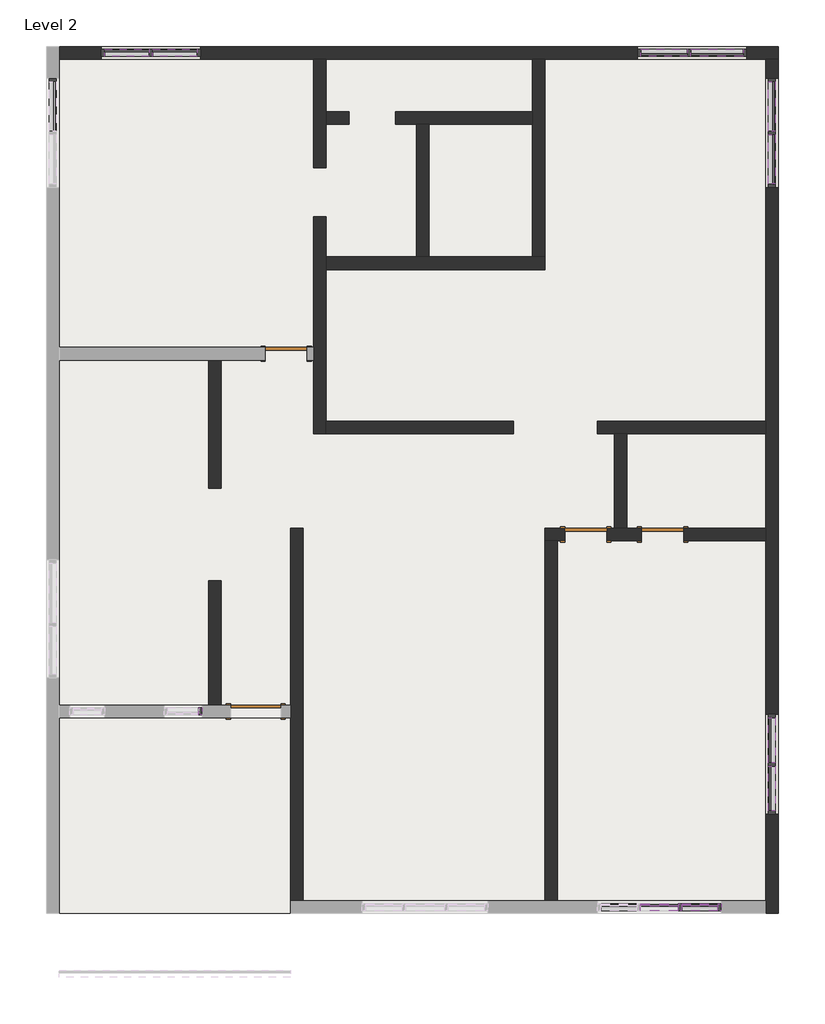
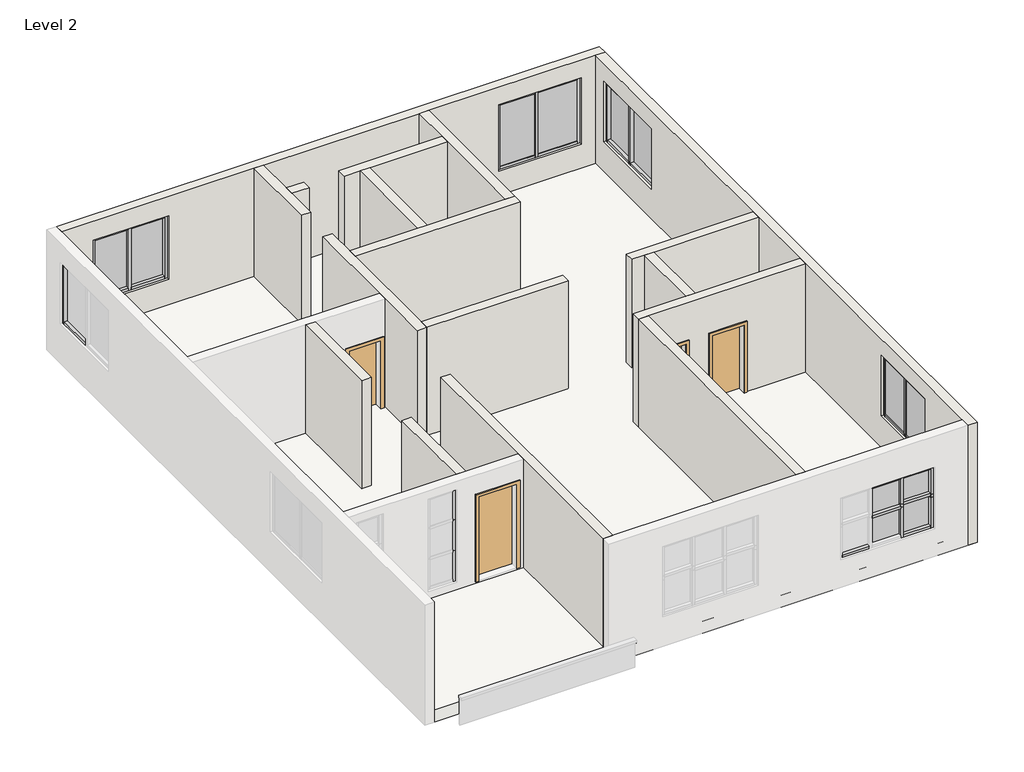
# One storey, part 2 of 2: 45 members, 17 walls, 12 plates, 4 doors, 1 roof.
"""IFC4 building model written with IfcOpenShell, lengths in millimetres."""

from ifc_helpers import new_model, si_unit, frame, origin, place, context, project, spatial, polyline, outline, extrude, faceted_brep, transform, mapped, element, save
from components import door_a1484949, door_85036156, door_0ca8825f, member_00d00b53, member_3d7cb871, member_933cb09f, member_c39a889e, member_9bd02798, member_f1f71bde, member_091e92f8, member_76c917ad, member_e74a93ea, member_cc8ff548, member_70242a31, member_df09edd1, member_4d9a94df, member_b41a733a, member_6d419de8, member_db897065, member_f4ec938c, member_27d1f1c9, member_a044dc63, member_e51dd2bd, member_dfbe4da1, member_32677b83, member_a37bde81, system_panel_glazed_bdc0238d, system_panel_glazed_a6d6e80d, system_panel_glazed_e66cc300, system_panel_glazed_239ce734, system_panel_glazed_acb18a83, system_panel_glazed_af458955, system_panel_glazed_d6f2290d, system_panel_glazed_2cf72723, system_panel_glazed_2eb886e8

model = new_model("IFC4")

# Units and contexts
model_context = context("Model", 3, world=origin())
ifc_project = project(units=[si_unit("LENGTHUNIT", "METRE", prefix="MILLI")], contexts=[model_context])

# Site, building, storey
site = spatial("IfcSite", under=ifc_project)
building = spatial("IfcBuilding", under=site)
storey = spatial("IfcBuildingStorey", under=building, Name="Level 2", Elevation=3048.0)

# Doors
placement = place(None, origin())
door_shape = door_a1484949(model_context)
element("IfcDoor", 1, ObjectType="Single-Flush : 30\" x 80\"", at=placement, inside=storey, context=model_context, shape_type="MappedRepresentation", body=[
    mapped(door_shape, transform((-14457.5127168, -4725.546149, 3048.0), x_axis=(1.0, 0.0, 0.0), y_axis=(0.0, 1.0, 0.0), z_axis=(0.0, 0.0, 1.0))),
])
element("IfcDoor", 2, ObjectType="Single-Flush : 30\" x 80\"", at=placement, inside=storey, context=model_context, shape_type="MappedRepresentation", body=[
    mapped(door_shape, transform((-9027.8261094, -8002.146149, 3048.0), x_axis=(1.0, 0.0, 0.0), y_axis=(0.0, 1.0, 0.0), z_axis=(0.0, 0.0, 1.0))),
])
door_2_shape = door_85036156(model_context)
element("IfcDoor", 3, ObjectType="Single-Flush : 30\" x 80\"", at=placement, inside=storey, context=model_context, shape_type="MappedRepresentation", body=[
    mapped(door_2_shape, transform((-7637.1761094, -8002.146149, 3048.0), x_axis=(-1.0, 0.0, 0.0), y_axis=(0.0, -1.0, 0.0), z_axis=(0.0, 0.0, 1.0))),
])
door_3_shape = door_0ca8825f(model_context)
element("IfcDoor", 4, ObjectType="Single-Flush : 36\" x 84\"", at=placement, inside=storey, context=model_context, shape_type="MappedRepresentation", body=[
    mapped(door_3_shape, transform((-15009.5261094, -11202.546149, 3403.6), x_axis=(1.0, 0.0, 0.0), y_axis=(0.0, 1.0, 0.0), z_axis=(0.0, 0.0, 1.0))),
])

# Members
member_shape = member_00d00b53(model_context)
element("IfcMember", 5, ObjectType="Rectangular Mullion : 2.5\" x 5\" rectangular", at=placement, inside=storey, context=model_context, shape_type="MappedRepresentation", body=[
    mapped(member_shape, transform((-7319.8216452, -14745.846149, 4532.9555732), x_axis=(1.0, 0.0, 0.0), y_axis=(0.0, -1.0, 0.0), z_axis=(0.0, 0.0, -1.0))),
])
member_2_shape = member_3d7cb871(model_context)
element("IfcMember", 6, ObjectType="Rectangular Mullion : 2.5\" x 5\" rectangular", at=placement, inside=storey, context=model_context, shape_type="MappedRepresentation", body=[
    mapped(member_2_shape, transform((-6570.3761094, -14745.846149, 4532.9555732), x_axis=(1.0, 0.0, 0.0), y_axis=(0.0, -1.0, 0.0), z_axis=(0.0, 0.0, -1.0))),
])
member_3_shape = member_933cb09f(model_context)
element("IfcMember", 7, ObjectType="Rectangular Mullion : 2.5\" x 5\" rectangular", at=placement, inside=storey, context=model_context, shape_type="MappedRepresentation", body=[
    mapped(member_3_shape, transform((-5655.9761094, -12194.7225944, 5677.6081175), x_axis=(0.0, 0.0, 1.0), y_axis=(1.0, 0.0, 0.0), z_axis=(0.0, 1.0, 0.0))),
])
element("IfcMember", 8, ObjectType="Rectangular Mullion : 2.5\" x 5\" rectangular", at=placement, inside=storey, context=model_context, shape_type="MappedRepresentation", body=[
    mapped(member_3_shape, transform((-5655.9761094, -11319.9990397, 5677.6081175), x_axis=(0.0, 0.0, 1.0), y_axis=(1.0, 0.0, 0.0), z_axis=(0.0, 1.0, 0.0))),
])
member_4_shape = member_c39a889e(model_context)
element("IfcMember", 9, ObjectType="Rectangular Mullion : 2.5\" x 5\" rectangular", at=placement, inside=storey, context=model_context, shape_type="MappedRepresentation", body=[
    mapped(member_4_shape, transform((-5655.9761094, -12162.9725944, 4144.9262175), x_axis=(0.0, 1.0, 0.0), y_axis=(1.0, 0.0, 0.0), z_axis=(0.0, 0.0, -1.0))),
])
element("IfcMember", 10, ObjectType="Rectangular Mullion : 2.5\" x 5\" rectangular", at=placement, inside=storey, context=model_context, shape_type="MappedRepresentation", body=[
    mapped(member_4_shape, transform((-5655.9761094, -725.046149, 4111.8628556), x_axis=(0.0, -1.0, 0.0), y_axis=(-1.0, 0.0, 0.0), z_axis=(0.0, 0.0, -1.0))),
])
element("IfcMember", 11, ObjectType="Rectangular Mullion : 2.5\" x 5\" rectangular", at=placement, inside=storey, context=model_context, shape_type="MappedRepresentation", body=[
    mapped(member_3_shape, transform((-5655.9761094, -12131.2225944, 4144.9262175), x_axis=(0.0, 0.0, -1.0), y_axis=(1.0, 0.0, 0.0), z_axis=(0.0, -1.0, 0.0))),
])
element("IfcMember", 12, ObjectType="Rectangular Mullion : 2.5\" x 5\" rectangular", at=placement, inside=storey, context=model_context, shape_type="MappedRepresentation", body=[
    mapped(member_3_shape, transform((-5655.9761094, -13005.946149, 4144.9262175), x_axis=(0.0, 0.0, -1.0), y_axis=(1.0, 0.0, 0.0), z_axis=(0.0, -1.0, 0.0))),
])
member_5_shape = member_9bd02798(model_context)
element("IfcMember", 13, ObjectType="Rectangular Mullion : 2.5\" x 5\" rectangular", at=placement, inside=storey, context=model_context, shape_type="MappedRepresentation", body=[
    mapped(member_5_shape, transform((-5655.9761094, -11256.4990397, 4144.9262175), x_axis=(0.0, 1.0, 0.0), y_axis=(1.0, 0.0, 0.0), z_axis=(0.0, 0.0, -1.0))),
])
element("IfcMember", 14, ObjectType="Rectangular Mullion : 2.5\" x 5\" rectangular", at=placement, inside=storey, context=model_context, shape_type="MappedRepresentation", body=[
    mapped(member_5_shape, transform((-5655.9761094, -1715.646149, 4111.8628556), x_axis=(0.0, -1.0, 0.0), y_axis=(-1.0, 0.0, 0.0), z_axis=(0.0, 0.0, -1.0))),
])
element("IfcMember", 15, ObjectType="Rectangular Mullion : 2.5\" x 5\" rectangular", at=placement, inside=storey, context=model_context, shape_type="MappedRepresentation", body=[
    mapped(member_5_shape, transform((-5655.9761094, -13069.446149, 5677.6081175), x_axis=(0.0, -1.0, 0.0), y_axis=(1.0, 0.0, 0.0), z_axis=(0.0, 0.0, 1.0))),
])
element("IfcMember", 16, ObjectType="Rectangular Mullion : 2.5\" x 5\" rectangular", at=placement, inside=storey, context=model_context, shape_type="MappedRepresentation", body=[
    mapped(member_5_shape, transform((-5655.9761094, 265.553851, 5644.5447557), x_axis=(0.0, 1.0, 0.0), y_axis=(-1.0, 0.0, 0.0), z_axis=(0.0, 0.0, 1.0))),
])
member_6_shape = member_f1f71bde(model_context)
element("IfcMember", 17, ObjectType="Rectangular Mullion : 2.5\" x 5\" rectangular", at=placement, inside=storey, context=model_context, shape_type="MappedRepresentation", body=[
    mapped(member_6_shape, transform((-5655.9761094, -756.796149, 4111.8628556), x_axis=(0.0, 0.0, -1.0), y_axis=(-1.0, 0.0, 0.0), z_axis=(0.0, 1.0, 0.0))),
])
element("IfcMember", 18, ObjectType="Rectangular Mullion : 2.5\" x 5\" rectangular", at=placement, inside=storey, context=model_context, shape_type="MappedRepresentation", body=[
    mapped(member_6_shape, transform((-5655.9761094, 202.053851, 4111.8628556), x_axis=(0.0, 0.0, -1.0), y_axis=(-1.0, 0.0, 0.0), z_axis=(0.0, 1.0, 0.0))),
])
element("IfcMember", 19, ObjectType="Rectangular Mullion : 2.5\" x 5\" rectangular", at=placement, inside=storey, context=model_context, shape_type="MappedRepresentation", body=[
    mapped(member_6_shape, transform((-18686.1761094, 202.053851, 4059.4675701), x_axis=(0.0, 0.0, -1.0), y_axis=(-1.0, 0.0, 0.0), z_axis=(0.0, 1.0, 0.0))),
])
element("IfcMember", 20, ObjectType="Rectangular Mullion : 2.5\" x 5\" rectangular", at=placement, inside=storey, context=model_context, shape_type="MappedRepresentation", body=[
    mapped(member_6_shape, transform((-5655.9761094, -693.296149, 5644.5447557), x_axis=(0.0, 0.0, 1.0), y_axis=(-1.0, 0.0, 0.0), z_axis=(0.0, -1.0, 0.0))),
])
element("IfcMember", 21, ObjectType="Rectangular Mullion : 2.5\" x 5\" rectangular", at=placement, inside=storey, context=model_context, shape_type="MappedRepresentation", body=[
    mapped(member_6_shape, transform((-5655.9761094, -1652.146149, 5644.5447557), x_axis=(0.0, 0.0, 1.0), y_axis=(-1.0, 0.0, 0.0), z_axis=(0.0, -1.0, 0.0))),
])
member_7_shape = member_091e92f8(model_context)
element("IfcMember", 22, ObjectType="Rectangular Mullion : 2.5\" x 5\" rectangular", at=placement, inside=storey, context=model_context, shape_type="MappedRepresentation", body=[
    mapped(member_7_shape, transform((-8030.8761094, 722.753851, 5648.4248448), x_axis=(0.0, 0.0, 1.0), y_axis=(0.0, 1.0, 0.0), z_axis=(-1.0, 0.0, 0.0))),
])
member_8_shape = member_76c917ad(model_context)
element("IfcMember", 23, ObjectType="Rectangular Mullion : 2.5\" x 5\" rectangular", at=placement, inside=storey, context=model_context, shape_type="MappedRepresentation", body=[
    mapped(member_8_shape, transform((-7154.5761094, 722.753851, 3961.5338093), x_axis=(-1.0, 0.0, 0.0), y_axis=(0.0, 1.0, 0.0), z_axis=(0.0, 0.0, -1.0))),
])
element("IfcMember", 24, ObjectType="Rectangular Mullion : 2.5\" x 5\" rectangular", at=placement, inside=storey, context=model_context, shape_type="MappedRepresentation", body=[
    mapped(member_7_shape, transform((-7186.3261094, 722.753851, 3961.5338093), x_axis=(0.0, 0.0, -1.0), y_axis=(0.0, 1.0, 0.0), z_axis=(1.0, 0.0, 0.0))),
])
member_9_shape = member_e74a93ea(model_context)
element("IfcMember", 25, ObjectType="Rectangular Mullion : 2.5\" x 5\" rectangular", at=placement, inside=storey, context=model_context, shape_type="MappedRepresentation", body=[
    mapped(member_9_shape, transform((-8094.3761094, 722.753851, 3961.5338093), x_axis=(-1.0, 0.0, 0.0), y_axis=(0.0, 1.0, 0.0), z_axis=(0.0, 0.0, -1.0))),
])
member_10_shape = member_cc8ff548(model_context)
element("IfcMember", 26, ObjectType="Rectangular Mullion : 2.5\" x 5\" rectangular", at=placement, inside=storey, context=model_context, shape_type="MappedRepresentation", body=[
    mapped(member_10_shape, transform((-7122.8261094, 722.753851, 5648.4248448), x_axis=(0.0, 0.0, 1.0), y_axis=(0.0, 1.0, 0.0), z_axis=(-1.0, 0.0, 0.0))),
])
element("IfcMember", 27, ObjectType="Rectangular Mullion : 2.5\" x 5\" rectangular", at=placement, inside=storey, context=model_context, shape_type="MappedRepresentation", body=[
    mapped(member_10_shape, transform((-6176.6761094, 722.753851, 3961.5338093), x_axis=(0.0, 0.0, -1.0), y_axis=(0.0, 1.0, 0.0), z_axis=(1.0, 0.0, 0.0))),
])
element("IfcMember", 28, ObjectType="Rectangular Mullion : 2.5\" x 5\" rectangular", at=placement, inside=storey, context=model_context, shape_type="MappedRepresentation", body=[
    mapped(member_9_shape, transform((-6113.1761094, 722.753851, 5648.4248448), x_axis=(1.0, 0.0, 0.0), y_axis=(0.0, 1.0, 0.0), z_axis=(0.0, 0.0, 1.0))),
])
member_11_shape = member_70242a31(model_context)
element("IfcMember", 29, ObjectType="Rectangular Mullion : 2.5\" x 5\" rectangular", at=placement, inside=storey, context=model_context, shape_type="MappedRepresentation", body=[
    mapped(member_11_shape, transform((-16940.3627168, 722.753851, 5613.602116), x_axis=(0.0, 0.0, 1.0), y_axis=(0.0, -1.0, 0.0), z_axis=(1.0, 0.0, 0.0))),
])
element("IfcMember", 30, ObjectType="Rectangular Mullion : 2.5\" x 5\" rectangular", at=placement, inside=storey, context=model_context, shape_type="MappedRepresentation", body=[
    mapped(member_11_shape, transform((-16070.4127168, 722.753851, 5613.602116), x_axis=(0.0, 0.0, 1.0), y_axis=(0.0, -1.0, 0.0), z_axis=(1.0, 0.0, 0.0))),
])
member_12_shape = member_df09edd1(model_context)
element("IfcMember", 31, ObjectType="Rectangular Mullion : 2.5\" x 5\" rectangular", at=placement, inside=storey, context=model_context, shape_type="MappedRepresentation", body=[
    mapped(member_12_shape, transform((-16908.6127168, 722.753851, 4001.8843583), x_axis=(1.0, 0.0, 0.0), y_axis=(0.0, -1.0, 0.0), z_axis=(0.0, 0.0, -1.0))),
])
element("IfcMember", 32, ObjectType="Rectangular Mullion : 2.5\" x 5\" rectangular", at=placement, inside=storey, context=model_context, shape_type="MappedRepresentation", body=[
    mapped(member_11_shape, transform((-16876.8627168, 722.753851, 4001.8843583), x_axis=(0.0, 0.0, -1.0), y_axis=(0.0, -1.0, 0.0), z_axis=(-1.0, 0.0, 0.0))),
])
element("IfcMember", 33, ObjectType="Rectangular Mullion : 2.5\" x 5\" rectangular", at=placement, inside=storey, context=model_context, shape_type="MappedRepresentation", body=[
    mapped(member_11_shape, transform((-17746.8127168, 722.753851, 4001.8843583), x_axis=(0.0, 0.0, -1.0), y_axis=(0.0, -1.0, 0.0), z_axis=(-1.0, 0.0, 0.0))),
])
member_13_shape = member_4d9a94df(model_context)
element("IfcMember", 34, ObjectType="Rectangular Mullion : 2.5\" x 5\" rectangular", at=placement, inside=storey, context=model_context, shape_type="MappedRepresentation", body=[
    mapped(member_13_shape, transform((-17810.3127168, 722.753851, 5613.602116), x_axis=(-1.0, 0.0, 0.0), y_axis=(0.0, -1.0, 0.0), z_axis=(0.0, 0.0, 1.0))),
])
element("IfcMember", 35, ObjectType="Rectangular Mullion : 2.5\" x 5\" rectangular", at=placement, inside=storey, context=model_context, shape_type="MappedRepresentation", body=[
    mapped(member_13_shape, transform((-16006.9127168, 722.753851, 4001.8843583), x_axis=(1.0, 0.0, 0.0), y_axis=(0.0, -1.0, 0.0), z_axis=(0.0, 0.0, -1.0))),
])
member_14_shape = member_b41a733a(model_context)
element("IfcMember", 36, ObjectType="Rectangular Mullion : 2.5\" x 5\" rectangular", at=placement, inside=storey, context=model_context, shape_type="MappedRepresentation", body=[
    mapped(member_14_shape, transform((-18686.1761094, 265.553851, 5599.1263641), x_axis=(0.0, 1.0, 0.0), y_axis=(-1.0, 0.0, 0.0), z_axis=(0.0, 0.0, 1.0))),
])
member_15_shape = member_6d419de8(model_context)
element("IfcMember", 37, ObjectType="Rectangular Mullion : 2.5\" x 5\" rectangular", at=placement, inside=storey, context=model_context, shape_type="MappedRepresentation", body=[
    mapped(member_15_shape, transform((-15981.0761094, -11202.546149, 5884.8075695), x_axis=(1.0, 0.0, 0.0), y_axis=(0.0, 1.0, 0.0), z_axis=(0.0, 0.0, 1.0))),
])
element("IfcMember", 38, ObjectType="Rectangular Mullion : 2.5\" x 5\" rectangular", at=placement, inside=storey, context=model_context, shape_type="MappedRepresentation", body=[
    mapped(member_15_shape, transform((-15981.0761094, -11202.546149, 5104.8752687), x_axis=(1.0, 0.0, 0.0), y_axis=(0.0, 1.0, 0.0), z_axis=(0.0, 0.0, 1.0))),
])
element("IfcMember", 39, ObjectType="Rectangular Mullion : 2.5\" x 5\" rectangular", at=placement, inside=storey, context=model_context, shape_type="MappedRepresentation", body=[
    mapped(member_15_shape, transform((-15981.0761094, -11202.546149, 4324.942968), x_axis=(1.0, 0.0, 0.0), y_axis=(0.0, 1.0, 0.0), z_axis=(0.0, 0.0, 1.0))),
])
member_16_shape = member_db897065(model_context)
element("IfcMember", 40, ObjectType="Rectangular Mullion : 2.5\" x 5\" rectangular", at=placement, inside=storey, context=model_context, shape_type="MappedRepresentation", body=[
    mapped(member_16_shape, transform((-7319.8216452, -14745.846149, 4609.1555732), x_axis=(1.0, 0.0, 0.0), y_axis=(0.0, -1.0, 0.0), z_axis=(0.0, 0.0, -1.0))),
])
member_17_shape = member_f4ec938c(model_context)
element("IfcMember", 41, ObjectType="Rectangular Mullion : 2.5\" x 5\" rectangular", at=placement, inside=storey, context=model_context, shape_type="MappedRepresentation", body=[
    mapped(member_17_shape, transform((-7351.5716452, -14745.846149, 5311.3816242), x_axis=(0.0, 0.0, 1.0), y_axis=(0.0, -1.0, 0.0), z_axis=(1.0, 0.0, 0.0))),
])
member_18_shape = member_27d1f1c9(model_context)
element("IfcMember", 42, ObjectType="Rectangular Mullion : 2.5\" x 5\" rectangular", at=placement, inside=storey, context=model_context, shape_type="MappedRepresentation", body=[
    mapped(member_18_shape, transform((-7351.5716452, -14745.846149, 4532.9555732), x_axis=(0.0, 0.0, 1.0), y_axis=(0.0, -1.0, 0.0), z_axis=(1.0, 0.0, 0.0))),
])
member_19_shape = member_a044dc63(model_context)
element("IfcMember", 43, ObjectType="Rectangular Mullion : 2.5\" x 5\" rectangular", at=placement, inside=storey, context=model_context, shape_type="MappedRepresentation", body=[
    mapped(member_19_shape, transform((-6633.8761094, -14745.846149, 5311.3816242), x_axis=(0.0, 0.0, 1.0), y_axis=(0.0, -1.0, 0.0), z_axis=(1.0, 0.0, 0.0))),
])
member_20_shape = member_e51dd2bd(model_context)
element("IfcMember", 44, ObjectType="Rectangular Mullion : 2.5\" x 5\" rectangular", at=placement, inside=storey, context=model_context, shape_type="MappedRepresentation", body=[
    mapped(member_20_shape, transform((-6633.8761094, -14745.846149, 4609.1555732), x_axis=(0.0, 0.0, 1.0), y_axis=(0.0, -1.0, 0.0), z_axis=(1.0, 0.0, 0.0))),
])
member_21_shape = member_dfbe4da1(model_context)
element("IfcMember", 45, ObjectType="Rectangular Mullion : 2.5\" x 5\" rectangular", at=placement, inside=storey, context=model_context, shape_type="MappedRepresentation", body=[
    mapped(member_21_shape, transform((-6570.3761094, -14745.846149, 4609.1555732), x_axis=(1.0, 0.0, 0.0), y_axis=(0.0, -1.0, 0.0), z_axis=(0.0, 0.0, -1.0))),
])
member_22_shape = member_32677b83(model_context)
element("IfcMember", 46, ObjectType="Rectangular Mullion : 2.5\" x 5\" rectangular", at=placement, inside=storey, context=model_context, shape_type="MappedRepresentation", body=[
    mapped(member_22_shape, transform((-7319.8216452, -14745.846149, 3754.5295223), x_axis=(1.0, 0.0, 0.0), y_axis=(0.0, -1.0, 0.0), z_axis=(0.0, 0.0, -1.0))),
])
element("IfcMember", 47, ObjectType="Rectangular Mullion : 2.5\" x 5\" rectangular", at=placement, inside=storey, context=model_context, shape_type="MappedRepresentation", body=[
    mapped(member_19_shape, transform((-7288.0716452, -14745.846149, 3754.5295223), x_axis=(0.0, 0.0, -1.0), y_axis=(0.0, -1.0, 0.0), z_axis=(-1.0, 0.0, 0.0))),
])
element("IfcMember", 48, ObjectType="Rectangular Mullion : 2.5\" x 5\" rectangular", at=placement, inside=storey, context=model_context, shape_type="MappedRepresentation", body=[
    mapped(member_19_shape, transform((-8755.2127168, -14745.846149, 3754.5295223), x_axis=(0.0, 0.0, -1.0), y_axis=(0.0, -1.0, 0.0), z_axis=(-1.0, 0.0, 0.0))),
])
member_23_shape = member_a37bde81(model_context)
element("IfcMember", 49, ObjectType="Rectangular Mullion : 2.5\" x 5\" rectangular", at=placement, inside=storey, context=model_context, shape_type="MappedRepresentation", body=[
    mapped(member_23_shape, transform((-6570.3761094, -14745.846149, 3754.5295223), x_axis=(1.0, 0.0, 0.0), y_axis=(0.0, -1.0, 0.0), z_axis=(0.0, 0.0, -1.0))),
])

# Plates
system_panel_glazed_shape = system_panel_glazed_bdc0238d(model_context)
element("IfcPlate", 50, ObjectType="System Panel : Glazed", at=placement, inside=storey, context=model_context, shape_type="MappedRepresentation", body=[
    mapped(system_panel_glazed_shape, transform((-5655.9761094, -12600.3343717, 4208.4262175), x_axis=(0.0, 1.0, 0.0), y_axis=(-1.0, 0.0, 0.0), z_axis=(0.0, 0.0, 1.0))),
])
element("IfcPlate", 51, ObjectType="System Panel : Glazed", at=placement, inside=storey, context=model_context, shape_type="MappedRepresentation", body=[
    mapped(system_panel_glazed_shape, transform((-5655.9761094, -11725.610817, 4208.4262175), x_axis=(0.0, 1.0, 0.0), y_axis=(-1.0, 0.0, 0.0), z_axis=(0.0, 0.0, 1.0))),
])
system_panel_glazed_2_shape = system_panel_glazed_a6d6e80d(model_context)
element("IfcPlate", 52, ObjectType="System Panel : Glazed", at=placement, inside=storey, context=model_context, shape_type="MappedRepresentation", body=[
    mapped(system_panel_glazed_2_shape, transform((-5655.9761094, -245.621149, 4175.3628556), x_axis=(0.0, -1.0, 0.0), y_axis=(1.0, 0.0, 0.0), z_axis=(0.0, 0.0, 1.0))),
])
element("IfcPlate", 53, ObjectType="System Panel : Glazed", at=placement, inside=storey, context=model_context, shape_type="MappedRepresentation", body=[
    mapped(system_panel_glazed_2_shape, transform((-5655.9761094, -1204.471149, 4175.3628556), x_axis=(0.0, -1.0, 0.0), y_axis=(1.0, 0.0, 0.0), z_axis=(0.0, 0.0, 1.0))),
])
system_panel_glazed_3_shape = system_panel_glazed_e66cc300(model_context)
element("IfcPlate", 54, ObjectType="System Panel : Glazed", at=placement, inside=storey, context=model_context, shape_type="MappedRepresentation", body=[
    mapped(system_panel_glazed_3_shape, transform((-7608.6011094, 722.753851, 4025.0338093), x_axis=(-1.0, 0.0, 0.0), y_axis=(0.0, -1.0, 0.0), z_axis=(0.0, 0.0, 1.0))),
])
system_panel_glazed_4_shape = system_panel_glazed_239ce734(model_context)
element("IfcPlate", 55, ObjectType="System Panel : Glazed", at=placement, inside=storey, context=model_context, shape_type="MappedRepresentation", body=[
    mapped(system_panel_glazed_4_shape, transform((-6649.7511094, 722.753851, 4025.0338093), x_axis=(-1.0, 0.0, 0.0), y_axis=(0.0, -1.0, 0.0), z_axis=(0.0, 0.0, 1.0))),
])
system_panel_glazed_5_shape = system_panel_glazed_acb18a83(model_context)
element("IfcPlate", 56, ObjectType="System Panel : Glazed", at=placement, inside=storey, context=model_context, shape_type="MappedRepresentation", body=[
    mapped(system_panel_glazed_5_shape, transform((-17343.5877168, 722.753851, 4065.3843583), x_axis=(1.0, 0.0, 0.0), y_axis=(0.0, 1.0, 0.0), z_axis=(0.0, 0.0, 1.0))),
])
element("IfcPlate", 57, ObjectType="System Panel : Glazed", at=placement, inside=storey, context=model_context, shape_type="MappedRepresentation", body=[
    mapped(system_panel_glazed_5_shape, transform((-16473.6377168, 722.753851, 4065.3843583), x_axis=(1.0, 0.0, 0.0), y_axis=(0.0, 1.0, 0.0), z_axis=(0.0, 0.0, 1.0))),
])
system_panel_glazed_6_shape = system_panel_glazed_af458955(model_context)
element("IfcPlate", 58, ObjectType="System Panel : Glazed", at=placement, inside=storey, context=model_context, shape_type="MappedRepresentation", body=[
    mapped(system_panel_glazed_6_shape, transform((-7694.5444131, -14745.846149, 4564.7055732), x_axis=(1.0, 0.0, 0.0), y_axis=(0.0, 1.0, 0.0), z_axis=(0.0, 0.0, 1.0))),
])
system_panel_glazed_7_shape = system_panel_glazed_d6f2290d(model_context)
element("IfcPlate", 59, ObjectType="System Panel : Glazed", at=placement, inside=storey, context=model_context, shape_type="MappedRepresentation", body=[
    mapped(system_panel_glazed_7_shape, transform((-6960.9738773, -14745.846149, 4640.9055732), x_axis=(1.0, 0.0, 0.0), y_axis=(0.0, 1.0, 0.0), z_axis=(0.0, 0.0, 1.0))),
])
system_panel_glazed_8_shape = system_panel_glazed_2cf72723(model_context)
element("IfcPlate", 60, ObjectType="System Panel : Glazed", at=placement, inside=storey, context=model_context, shape_type="MappedRepresentation", body=[
    mapped(system_panel_glazed_8_shape, transform((-6960.9738773, -14745.846149, 3818.0295223), x_axis=(1.0, 0.0, 0.0), y_axis=(0.0, 1.0, 0.0), z_axis=(0.0, 0.0, 1.0))),
])
system_panel_glazed_9_shape = system_panel_glazed_2eb886e8(model_context)
element("IfcPlate", 61, ObjectType="System Panel : Glazed", at=placement, inside=storey, context=model_context, shape_type="MappedRepresentation", body=[
    mapped(system_panel_glazed_9_shape, transform((-7694.5444131, -14745.846149, 3818.0295223), x_axis=(1.0, 0.0, 0.0), y_axis=(0.0, 1.0, 0.0), z_axis=(0.0, 0.0, 1.0))),
])

# Roof
element("IfcRoof", 62, ObjectType="Generic - 12\"", at=placement, inside=storey, context=model_context, shape_type="SweptSolid", body=[
    extrude(outline(polyline([(-18800.4761094, 837.053851), (-5541.6761094, 837.053851), (-5541.6761094, -14860.146149), (-18800.4761094, -14860.146149), (-18800.4761094, 837.053851)])), frame((0.0, 0.0, 3048.0), z_axis=(0.0, 0.0, 1.0), x_axis=(1.0, 0.0, 0.0)), (0.0, 0.0, 1.0), 304.8),
])

# Walls
element("IfcWall", 63, ObjectType="9\"", at=placement, inside=storey, context=model_context, shape_type="Brep", body=[
    faceted_brep([(-18571.8761094, 608.453851, 3048.0), (-13962.2127168, 608.453851, 3048.0), (-13733.6127168, 608.453851, 3048.0), (-9999.3761094, 608.453851, 3048.0), (-9770.7761094, 608.453851, 3048.0), (-5770.2761094, 608.453851, 3048.0), (-5541.6761094, 608.453851, 3048.0), (-5541.6761094, 608.453851, 6096.0), (-5770.2761094, 608.453851, 6096.0), (-9770.7761094, 608.453851, 6096.0), (-9999.3761094, 608.453851, 6096.0), (-13733.6127168, 608.453851, 6096.0), (-13962.2127168, 608.453851, 6096.0), (-18571.8761094, 608.453851, 6096.0), (-17810.3127168, 608.453851, 4001.8843583), (-17810.3127168, 608.453851, 5613.602116), (-16006.9127168, 608.453851, 5613.602116), (-16006.9127168, 608.453851, 4001.8843583), (-6113.1761094, 608.453851, 5648.4248448), (-6113.1761094, 608.453851, 3961.5338093), (-8094.3761094, 608.453851, 3961.5338093), (-8094.3761094, 608.453851, 5648.4248448), (-5541.6761094, 837.053851, 3048.0), (-18571.8761094, 837.053851, 3048.0), (-18571.8761094, 837.053851, 6096.0), (-5541.6761094, 837.053851, 6096.0), (-17810.3127168, 837.053851, 5613.602116), (-17810.3127168, 837.053851, 4001.8843583), (-16006.9127168, 837.053851, 4001.8843583), (-16006.9127168, 837.053851, 5613.602116), (-6113.1761094, 837.053851, 3961.5338093), (-6113.1761094, 837.053851, 5648.4248448), (-8094.3761094, 837.053851, 5648.4248448), (-8094.3761094, 837.053851, 3961.5338093)], [[[0, 1, 2, 3, 4, 5, 6, 7, 8, 9, 10, 11, 12, 13], [14, 15, 16, 17], [18, 19, 20, 21]], [[22, 23, 24, 25], [26, 27, 28, 29], [30, 31, 32, 33]], [[6, 5, 4, 3, 2, 1, 0, 23, 22]], [[13, 12, 11, 10, 9, 8, 7, 25, 24]], [[0, 13, 24, 23]], [[7, 6, 22, 25]], [[14, 27, 26, 15]], [[15, 26, 29, 16]], [[16, 29, 28, 17]], [[27, 14, 17, 28]], [[30, 19, 18, 31]], [[31, 18, 21, 32]], [[20, 33, 32, 21]], [[19, 30, 33, 20]]]),
])
element("IfcWall", 64, ObjectType="9\"", at=placement, inside=storey, context=model_context, shape_type="Brep", body=[
    faceted_brep([(-5770.2761094, 608.453851, 3048.0), (-5770.2761094, -5944.746149, 3048.0), (-5770.2761094, -6173.346149, 3048.0), (-5770.2761094, -7887.846149, 3048.0), (-5770.2761094, -8116.446149, 3048.0), (-5770.2761094, -14631.546149, 3048.0), (-5770.2761094, -14860.146149, 3048.0), (-5770.2761094, -14860.146149, 6096.0), (-5770.2761094, -14631.546149, 6096.0), (-5770.2761094, -8116.446149, 6096.0), (-5770.2761094, -7887.846149, 6096.0), (-5770.2761094, -6173.346149, 6096.0), (-5770.2761094, -5944.746149, 6096.0), (-5770.2761094, 608.453851, 6096.0), (-5770.2761094, -13069.446149, 5677.6081175), (-5770.2761094, -13069.446149, 4144.9262175), (-5770.2761094, -11256.4990397, 4144.9262175), (-5770.2761094, -11256.4990397, 5677.6081175), (-5770.2761094, 265.553851, 4111.8628556), (-5770.2761094, 265.553851, 5644.5447557), (-5770.2761094, -1715.646149, 5644.5447557), (-5770.2761094, -1715.646149, 4111.8628556), (-5541.6761094, -14860.146149, 3048.0), (-5541.6761094, 608.453851, 3048.0), (-5541.6761094, 608.453851, 6096.0), (-5541.6761094, -14860.146149, 6096.0), (-5541.6761094, -13069.446149, 4144.9262175), (-5541.6761094, -13069.446149, 5677.6081175), (-5541.6761094, -11256.4990397, 5677.6081175), (-5541.6761094, -11256.4990397, 4144.9262175), (-5541.6761094, 265.553851, 5644.5447557), (-5541.6761094, 265.553851, 4111.8628556), (-5541.6761094, -1715.646149, 4111.8628556), (-5541.6761094, -1715.646149, 5644.5447557)], [[[0, 1, 2, 3, 4, 5, 6, 7, 8, 9, 10, 11, 12, 13], [14, 15, 16, 17], [18, 19, 20, 21]], [[22, 23, 24, 25], [26, 27, 28, 29], [30, 31, 32, 33]], [[6, 5, 4, 3, 2, 1, 0, 23, 22]], [[13, 12, 11, 10, 9, 8, 7, 25, 24]], [[0, 13, 24, 23]], [[7, 6, 22, 25]], [[26, 15, 14, 27]], [[27, 14, 17, 28]], [[16, 29, 28, 17]], [[15, 26, 29, 16]], [[18, 31, 30, 19]], [[19, 30, 33, 20]], [[20, 33, 32, 21]], [[31, 18, 21, 32]]]),
])
element("IfcWall", 65, ObjectType="9\"", at=placement, inside=storey, context=model_context, shape_type="Brep", body=[
    faceted_brep([(-14380.8761094, -7887.846149, 3048.0), (-14380.8761094, -11088.246149, 3048.0), (-14380.8761094, -11316.846149, 3048.0), (-14380.8761094, -14631.546149, 3048.0), (-14380.8761094, -14631.546149, 6096.0), (-14380.8761094, -11316.846149, 6096.0), (-14380.8761094, -11088.246149, 6096.0), (-14380.8761094, -7887.846149, 6096.0), (-14152.2761094, -7887.846149, 3048.0), (-14152.2761094, -7887.846149, 6096.0), (-14152.2761094, -14631.546149, 6096.0), (-14152.2761094, -14631.546149, 3048.0)], [[[0, 1, 2, 3, 4, 5, 6, 7]], [[8, 9, 10, 11]], [[3, 2, 1, 0, 8, 11]], [[7, 6, 5, 4, 10, 9]], [[0, 7, 9, 8]], [[4, 3, 11, 10]]]),
])
element("IfcWall", 66, ObjectType="9\"", at=placement, inside=storey, context=model_context, shape_type="SweptSolid", body=[
    extrude(outline(polyline([(-15866.7761094, -11088.246149), (-15866.7761094, -8840.346149), (-15638.1761094, -8840.346149), (-15638.1761094, -11088.246149), (-15866.7761094, -11088.246149)])), frame((0.0, 0.0, 3048.0), z_axis=(0.0, 0.0, 1.0), x_axis=(1.0, 0.0, 0.0)), (0.0, 0.0, 1.0), 3048.0),
])
element("IfcWall", 67, ObjectType="9\"", at=placement, inside=storey, context=model_context, shape_type="Brep", body=[
    faceted_brep([(-13733.6127168, -6173.346149, 3048.0), (-13733.6127168, -5944.746149, 3048.0), (-13733.6127168, -3201.546149, 3048.0), (-13733.6127168, -2972.946149, 3048.0), (-13733.6127168, -2249.046149, 3048.0), (-13733.6127168, -2249.046149, 6096.0), (-13733.6127168, -2972.946149, 6096.0), (-13733.6127168, -3201.546149, 6096.0), (-13733.6127168, -5944.746149, 6096.0), (-13733.6127168, -6173.346149, 6096.0), (-13962.2127168, -6173.346149, 3048.0), (-13962.2127168, -6173.346149, 6096.0), (-13962.2127168, -4839.846149, 6096.0), (-13962.2127168, -4611.246149, 6096.0), (-13962.2127168, -2249.046149, 6096.0), (-13962.2127168, -2249.046149, 3048.0), (-13962.2127168, -4611.246149, 3048.0), (-13962.2127168, -4839.846149, 3048.0)], [[[0, 1, 2, 3, 4, 5, 6, 7, 8, 9]], [[10, 11, 12, 13, 14, 15, 16, 17]], [[4, 3, 2, 1, 0, 10, 17, 16, 15]], [[5, 4, 15, 14]], [[9, 8, 7, 6, 5, 14, 13, 12, 11]], [[0, 9, 11, 10]]]),
])
element("IfcWall", 68, ObjectType="9\"", at=placement, inside=storey, context=model_context, shape_type="Brep", body=[
    faceted_brep([(-13733.6127168, -3201.546149, 3048.0), (-9770.7761094, -3201.546149, 3048.0), (-9770.7761094, -3201.546149, 6096.0), (-13733.6127168, -3201.546149, 6096.0), (-13733.6127168, -2972.946149, 3048.0), (-13733.6127168, -2972.946149, 6096.0), (-12095.0944131, -2972.946149, 6096.0), (-11866.4944131, -2972.946149, 6096.0), (-9999.3761094, -2972.946149, 6096.0), (-9770.7761094, -2972.946149, 6096.0), (-9770.7761094, -2972.946149, 3048.0), (-9999.3761094, -2972.946149, 3048.0), (-11866.4944131, -2972.946149, 3048.0), (-12095.0944131, -2972.946149, 3048.0)], [[[0, 1, 2, 3]], [[4, 5, 6, 7, 8, 9, 10, 11, 12, 13]], [[1, 0, 4, 13, 12, 11, 10]], [[3, 2, 9, 8, 7, 6, 5]], [[0, 3, 5, 4]], [[2, 1, 10, 9]]]),
])
element("IfcWall", 69, ObjectType="9\"", at=placement, inside=storey, context=model_context, shape_type="Brep", body=[
    faceted_brep([(-9999.3761094, 608.453851, 3048.0), (-9999.3761094, -344.046149, 3048.0), (-9999.3761094, -572.646149, 3048.0), (-9999.3761094, -2972.946149, 3048.0), (-9999.3761094, -2972.946149, 6096.0), (-9999.3761094, -572.646149, 6096.0), (-9999.3761094, -344.046149, 6096.0), (-9999.3761094, 608.453851, 6096.0), (-9770.7761094, 608.453851, 3048.0), (-9770.7761094, 608.453851, 6096.0), (-9770.7761094, -2972.946149, 6096.0), (-9770.7761094, -2972.946149, 3048.0)], [[[0, 1, 2, 3, 4, 5, 6, 7]], [[8, 9, 10, 11]], [[3, 2, 1, 0, 8, 11]], [[7, 6, 5, 4, 10, 9]], [[4, 3, 11, 10]], [[0, 7, 9, 8]]]),
])
element("IfcWall", 70, ObjectType="9\"", at=placement, inside=storey, context=model_context, shape_type="Brep", body=[
    faceted_brep([(-12476.3127168, -572.646149, 3048.0), (-12095.0944131, -572.646149, 3048.0), (-11866.4944131, -572.646149, 3048.0), (-9999.3761094, -572.646149, 3048.0), (-9999.3761094, -572.646149, 6096.0), (-11866.4944131, -572.646149, 6096.0), (-12095.0944131, -572.646149, 6096.0), (-12476.3127168, -572.646149, 6096.0), (-12476.3127168, -344.046149, 3048.0), (-12476.3127168, -344.046149, 6096.0), (-9999.3761094, -344.046149, 6096.0), (-9999.3761094, -344.046149, 3048.0)], [[[0, 1, 2, 3, 4, 5, 6, 7]], [[8, 9, 10, 11]], [[3, 2, 1, 0, 8, 11]], [[7, 6, 5, 4, 10, 9]], [[0, 7, 9, 8]], [[4, 3, 11, 10]]]),
])
element("IfcWall", 71, ObjectType="9\"", at=placement, inside=storey, context=model_context, shape_type="SweptSolid", body=[
    extrude(outline(polyline([(-12095.0944131, -2972.946149), (-12095.0944131, -572.646149), (-11866.4944131, -572.646149), (-11866.4944131, -2972.946149), (-12095.0944131, -2972.946149)])), frame((0.0, 0.0, 3048.0), z_axis=(0.0, 0.0, 1.0), x_axis=(1.0, 0.0, 0.0)), (0.0, 0.0, 1.0), 3048.0),
])
element("IfcWall", 72, ObjectType="9\"", at=placement, inside=storey, context=model_context, shape_type="Brep", body=[
    faceted_brep([(-13962.2127168, 608.453851, 3048.0), (-13962.2127168, -1360.046149, 3048.0), (-13962.2127168, -1360.046149, 6096.0), (-13962.2127168, 608.453851, 6096.0), (-13733.6127168, 608.453851, 3048.0), (-13733.6127168, 608.453851, 6096.0), (-13733.6127168, -344.046149, 6096.0), (-13733.6127168, -572.646149, 6096.0), (-13733.6127168, -1360.046149, 6096.0), (-13733.6127168, -1360.046149, 3048.0), (-13733.6127168, -572.646149, 3048.0), (-13733.6127168, -344.046149, 3048.0)], [[[0, 1, 2, 3]], [[4, 5, 6, 7, 8, 9, 10, 11]], [[1, 0, 4, 11, 10, 9]], [[2, 1, 9, 8]], [[3, 2, 8, 7, 6, 5]], [[0, 3, 5, 4]]]),
])
element("IfcWall", 73, ObjectType="9\"", at=placement, inside=storey, context=model_context, shape_type="SweptSolid", body=[
    extrude(outline(polyline([(-13314.5127168, -572.646149), (-13733.6127168, -572.646149), (-13733.6127168, -344.046149), (-13314.5127168, -344.046149), (-13314.5127168, -572.646149)])), frame((0.0, 0.0, 3048.0), z_axis=(0.0, 0.0, 1.0), x_axis=(1.0, 0.0, 0.0)), (0.0, 0.0, 1.0), 3048.0),
])
element("IfcWall", 74, ObjectType="9\"", at=placement, inside=storey, context=model_context, shape_type="SweptSolid", body=[
    extrude(outline(polyline([(-15866.7761094, -7163.946149), (-15866.7761094, -4839.846149), (-15638.1761094, -4839.846149), (-15638.1761094, -7163.946149), (-15866.7761094, -7163.946149)])), frame((0.0, 0.0, 3048.0), z_axis=(0.0, 0.0, 1.0), x_axis=(1.0, 0.0, 0.0)), (0.0, 0.0, 1.0), 3048.0),
])
element("IfcWall", 75, ObjectType="9\"", at=placement, inside=storey, context=model_context, shape_type="SweptSolid", body=[
    extrude(outline(polyline([(-10342.7127168, -6173.346149), (-13733.6127168, -6173.346149), (-13733.6127168, -5944.746149), (-10342.7127168, -5944.746149), (-10342.7127168, -6173.346149)])), frame((0.0, 0.0, 3048.0), z_axis=(0.0, 0.0, 1.0), x_axis=(1.0, 0.0, 0.0)), (0.0, 0.0, 1.0), 3048.0),
])
element("IfcWall", 76, ObjectType="9\"", at=placement, inside=storey, context=model_context, shape_type="Brep", body=[
    faceted_brep([(-8818.7127168, -6173.346149, 3048.0), (-8513.4761094, -6173.346149, 3048.0), (-8284.8761094, -6173.346149, 3048.0), (-5770.2761094, -6173.346149, 3048.0), (-5770.2761094, -6173.346149, 6096.0), (-8284.8761094, -6173.346149, 6096.0), (-8513.4761094, -6173.346149, 6096.0), (-8818.7127168, -6173.346149, 6096.0), (-8818.7127168, -5944.746149, 3048.0), (-8818.7127168, -5944.746149, 6096.0), (-5770.2761094, -5944.746149, 6096.0), (-5770.2761094, -5944.746149, 3048.0)], [[[0, 1, 2, 3, 4, 5, 6, 7]], [[8, 9, 10, 11]], [[3, 2, 1, 0, 8, 11]], [[7, 6, 5, 4, 10, 9]], [[0, 7, 9, 8]], [[4, 3, 11, 10]]]),
])
element("IfcWall", 77, ObjectType="9\"", at=placement, inside=storey, context=model_context, shape_type="SweptSolid", body=[
    extrude(outline(polyline([(-8513.4761094, -7887.846149), (-8513.4761094, -6173.346149), (-8284.8761094, -6173.346149), (-8284.8761094, -7887.846149), (-8513.4761094, -7887.846149)])), frame((0.0, 0.0, 3048.0), z_axis=(0.0, 0.0, 1.0), x_axis=(1.0, 0.0, 0.0)), (0.0, 0.0, 1.0), 3048.0),
])
element("IfcWall", 78, ObjectType="9\"", at=placement, inside=storey, context=model_context, shape_type="Brep", body=[
    faceted_brep([(-8646.8261094, -8116.446149, 3048.0), (-8018.1761094, -8116.446149, 3048.0), (-8018.1761094, -8116.446149, 5080.0), (-7256.1761094, -8116.446149, 5080.0), (-7256.1761094, -8116.446149, 3048.0), (-5770.2761094, -8116.446149, 3048.0), (-5770.2761094, -8116.446149, 6096.0), (-9542.1761094, -8116.446149, 6096.0), (-9770.7761094, -8116.446149, 6096.0), (-9770.7761094, -8116.446149, 3048.0), (-9542.1761094, -8116.446149, 3048.0), (-9408.8261094, -8116.446149, 3048.0), (-9408.8261094, -8116.446149, 5080.0), (-8646.8261094, -8116.446149, 5080.0), (-8018.1761094, -7887.846149, 5080.0), (-8018.1761094, -7887.846149, 3048.0), (-8284.8761094, -7887.846149, 3048.0), (-8513.4761094, -7887.846149, 3048.0), (-8646.8261094, -7887.846149, 3048.0), (-8646.8261094, -7887.846149, 5080.0), (-9408.8261094, -7887.846149, 5080.0), (-9408.8261094, -7887.846149, 3048.0), (-9770.7761094, -7887.846149, 3048.0), (-9770.7761094, -7887.846149, 6096.0), (-8513.4761094, -7887.846149, 6096.0), (-8284.8761094, -7887.846149, 6096.0), (-5770.2761094, -7887.846149, 6096.0), (-5770.2761094, -7887.846149, 3048.0), (-7256.1761094, -7887.846149, 3048.0), (-7256.1761094, -7887.846149, 5080.0)], [[[0, 1, 2, 3, 4, 5, 6, 7, 8, 9, 10, 11, 12, 13]], [[14, 15, 16, 17, 18, 19, 20, 21, 22, 23, 24, 25, 26, 27, 28, 29]], [[11, 10, 9, 22, 21]], [[28, 27, 5, 4]], [[18, 17, 16, 15, 1, 0]], [[8, 7, 6, 26, 25, 24, 23]], [[6, 5, 27, 26]], [[9, 8, 23, 22]], [[19, 18, 0, 13]], [[20, 19, 13, 12]], [[21, 20, 12, 11]], [[2, 1, 15, 14]], [[3, 2, 14, 29]], [[4, 3, 29, 28]]]),
])
element("IfcWall", 79, ObjectType="9\"", at=placement, inside=storey, context=model_context, shape_type="SweptSolid", body=[
    extrude(outline(polyline([(-9770.7761094, -14631.546149), (-9770.7761094, -8116.446149), (-9542.1761094, -8116.446149), (-9542.1761094, -14631.546149), (-9770.7761094, -14631.546149)])), frame((0.0, 0.0, 3048.0), z_axis=(0.0, 0.0, 1.0), x_axis=(1.0, 0.0, 0.0)), (0.0, 0.0, 1.0), 3048.0),
])

save(model, "model.ifc")

# Revit data of these elements
# Type "Single-Flush : 30\" x 80\""
#   Type Mark = "5"
#   Construction Type Id = "MDOOR"
#   Assembly Code = "C1020"
#   Analytic Construction = "Metal"
#   Thickness = 0' - 2"
#   Heat Transfer Coefficient (U) = 0.651978 BTU/(h·ft²·°F)
#   Height = 6' - 8"
#   Trim Projection Ext = 0' - 1"
#   Trim Projection Int = 0' - 1"
#   Trim Width = 0' - 3"
#   Width = 2' - 6"
#   Define Thermal Properties by = 1
#   Define Thermal Properties by = 1
#   Door Material = Door - Panel
#   Frame Material = Door - Frame
#   Visual Light Transmittance = 0
#   Solar Heat Gain Coefficient = 0
#   Function = (empty or 0)
#   Wall Closure = (empty or 0)
# Type "Single-Flush : 36\" x 84\""
#   Type Mark = "1"
#   Construction Type Id = "MDOOR"
#   Assembly Code = "C1020"
#   Analytic Construction = "Metal"
#   Thickness = 0' - 2"
#   Heat Transfer Coefficient (U) = 0.651978 BTU/(h·ft²·°F)
#   Height = 7' - 0"
#   Trim Projection Ext = 0' - 1"
#   Trim Projection Int = 0' - 1"
#   Trim Width = 0' - 3"
#   Width = 3' - 0"
#   Define Thermal Properties by = 1
#   Define Thermal Properties by = 1
#   Door Material = Door - Panel
#   Frame Material = Door - Frame
#   Visual Light Transmittance = 0
#   Solar Heat Gain Coefficient = 0
#   Function = (empty or 0)
#   Wall Closure = (empty or 0)
# Type "Rectangular Mullion : 2.5\" x 5\" rectangular"
#   built-in parameter 1007304 = 0.416667 (stored number, unit not read)
#   built-in parameter 1007301 = 0.104167 (stored number, unit not read)
#   built-in parameter 1007300 = 0.104167 (stored number, unit not read)
# Type "System Panel : Glazed"
#   Construction Type Id = "GSP4R"
#   Analytic Construction = "1/8 in Pilkington single glazing"
#   Visual Light Transmittance = 0.9
#   Solar Heat Gain Coefficient = 0.86
#   Heat Transfer Coefficient (U) = 1.18115 BTU/(h·ft²·°F)
#   Define Thermal Properties by = 1
# Type "Generic - 12\""
#   Assembly Code = "B1020"
#   Layers, outside or top first: 1' - 0" no material (function 1)
# Type "9\""
#   Assembly Code = "B2010"
#   Layers, outside or top first: 0' - 9" no material (function 1)
# Elements 1, 2, 3 (IfcDoor, "Single-Flush : 30\" x 80\"")
#   Phase Created = New Construction
#   Materials on its faces: "Door - Frame", "Door - Panel"
# Element 4 (IfcDoor, "Single-Flush : 36\" x 84\"")
#   Phase Created = New Construction
#   Materials on its faces: "Door - Frame", "Door - Panel"
# Elements 5, 6, 7, 8, 9, 10, 11, 12, 13, 14, 15, 16, 17, 18, 19, 20, 21, 22, 23, 24, 25, 26, 27, 28, 29, 30, 31, 32, 33, 34, 35, 36, 37, 38, 39, 40, 41, 42, 43, 44, 45, 46, 47, 48, 49 (IfcMember, "Rectangular Mullion : 2.5\" x 5\" rectangular")
#   Phase Created = New Construction
#   Materials on its faces: "Aluminum"
# Elements 50, 51, 52, 53, 54, 55, 56, 57, 58, 59, 60, 61 (IfcPlate, "System Panel : Glazed")
#   Phase Created = New Construction
#   Materials on its faces: "Glass"
# Element 62 (IfcRoof, "Generic - 12\"")
#   built-in parameter 1001705 = 11 (stored number, unit not read)
#   built-in parameter 1001710 = 33615
#   Phase Created = New Construction
#   Materials on its faces: "Default Roof"
# Elements 63, 64, 65, 66, 67, 68, 69, 70, 71, 72, 73, 74, 75, 76, 77, 78, 79 (IfcWall, "9\"")
#   Top Offset = 0' - 0"
#   Base Offset = 0' - 0"
#   Unconnected Height = 10' - 0"
#   wall height = 10' - 0"
#   Phase Created = New Construction
#   Base Constraint = Level 2
#   Materials on its faces: "Default Wall"
# Materials
#   "Door - Panel": class "Wood", colour RGB 210 159 95, transparency 0, Cost = 0
#   "Door - Frame": colour RGB 118 70 51, transparency 0, Cost = 0
#   "Aluminum": class "Metal", colour RGB 247 247 247, transparency 0, Description = "Aluminum 6061", Cost = 0
#   "Glass": class "Glass", colour RGB 0 128 192, transparency 0.75, Description = "Soda Lime Glass", Cost = 0
#   "Default Roof": colour RGB 88 101 114, transparency 0, Cost = 0
#   "Default Wall": colour RGB 128 128 128, transparency 0, Cost = 0
